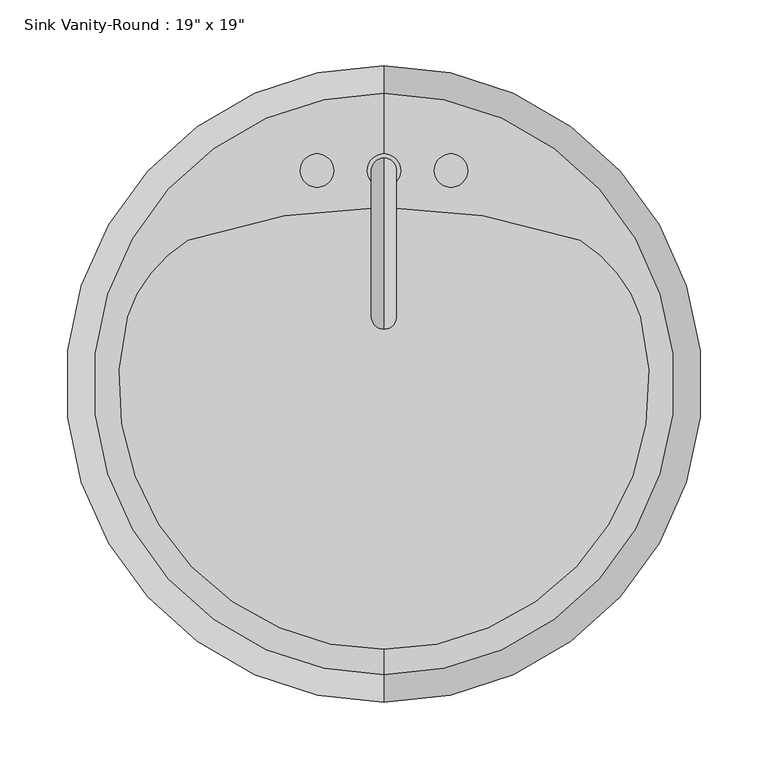
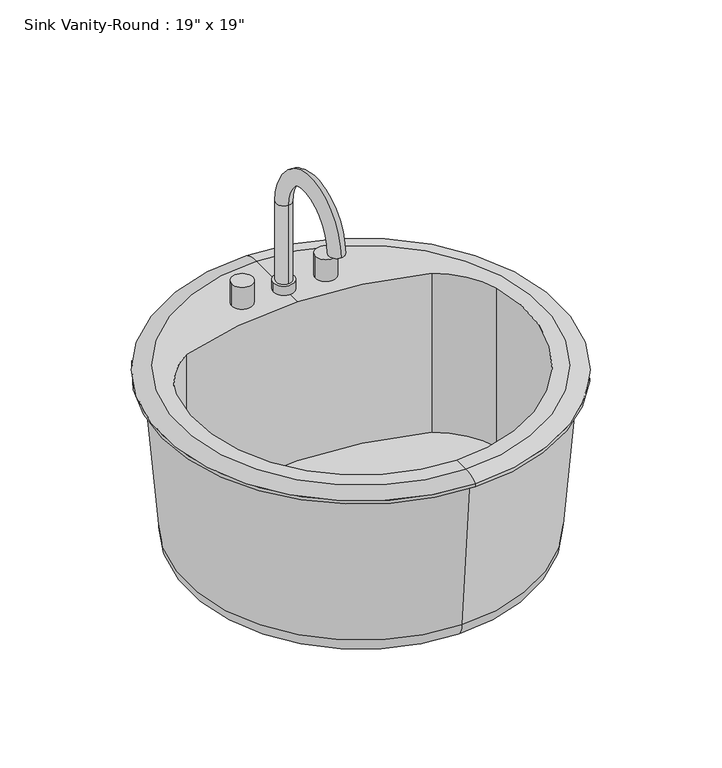
"""IFC4 building model written with IfcOpenShell, lengths in millimetres: flow terminal geometry."""

from ifc_helpers import new_model, si_unit, point, frame, frame_2d, origin, place, context, project, spatial, polyline, circle_curve, ellipse_curve, trimmed, segment, composite_curve, outline, extrude, source, transform, mapped, element, save
from ifc_brep_helpers import plane_surface, cylinder_surface, revolved_surface, advanced_brep


def flow_terminal_a43f4bde(model_context):
    return source(origin(), model_context, "Body", "SolidModel", [
        advanced_brep(
        [(96.6517406, -135.3870093, 796.925), (96.6517406, 305.7224463, 796.925), (96.6517406, 326.4677185, 791.36875), (96.6517406, -156.1322815, 791.36875), (96.6517406, -116.2405705, 796.925), (-98.1703414, 136.2525038, 796.925), (-52.1534933, 194.0861398, 796.925), (96.6517406, 219.2662048, 796.925), (245.4569744, 194.0861398, 796.925), (291.4738225, 136.2525038, 796.925), (96.6517406, -107.1264028, 571.5), (96.6517406, 277.4618398, 571.5), (96.6517406, 85.1677185, 571.5), (96.6517406, -127.6827361, 592.6842611), (96.6517406, 298.0181731, 592.6842611), (96.6517406, -144.2260315, 787.4), (96.6517406, 314.5614685, 787.4), (96.6517406, -156.1322815, 787.4), (96.6517406, 326.4677185, 787.4), (245.4569744, 194.0861398, 592.6842611), (-52.1534933, 194.0861398, 592.6842611), (-98.1703414, 136.2525038, 592.6842611), (291.4738225, 136.2525038, 592.6842611)],
        [
            (0, 1, circle_curve(frame((96.6517406, 85.1677185, 796.925), z_axis=(0.0, 0.0, -1.0), x_axis=(0.0, 1.0, 0.0)), 220.5547278)),
            (1, 2, circle_curve(frame((96.6517406, 309.4374616, 769.289434), z_axis=(-1.0, 0.0, 0.0), x_axis=(0.0, 1.0, 0.0)), 27.8841505)),
            (2, 3, circle_curve(frame((96.6517406, 85.1677185, 791.36875), z_axis=(0.0, 0.0, 1.0), x_axis=(0.0, 1.0, 0.0)), 241.3)),
            (3, 0, circle_curve(frame((96.6517406, -139.1020246, 769.289434), z_axis=(-1.0, 0.0, 0.0), x_axis=(0.0, -1.0, 0.0)), 27.8841505)),
            (1, 0, circle_curve(frame((96.6517406, 85.1677185, 796.925), z_axis=(0.0, 0.0, -1.0), x_axis=(0.0, 1.0, 0.0)), 220.5547278)),
            (3, 2, circle_curve(frame((96.6517406, 85.1677185, 791.36875), z_axis=(0.0, 0.0, 1.0), x_axis=(0.0, 1.0, 0.0)), 241.3)),
            (0, 4),
            (4, 5, circle_curve(frame((96.6517406, 85.1677185, 796.925), z_axis=(0.0, 0.0, -1.0), x_axis=(1.0, 0.0, 0.0)), 201.408289)),
            (5, 6, circle_curve(frame((1.3689689, 104.2755165, 796.925), z_axis=(0.0, 0.0, -1.0), x_axis=(1.0, 0.0, 0.0)), 104.5495194)),
            (6, 7, circle_curve(frame((96.6517406, -233.0168462, 796.925), z_axis=(0.0, 0.0, -1.0), x_axis=(1.0, 0.0, 0.0)), 452.283051)),
            (7, 1),
            (7, 8, circle_curve(frame((96.6517406, -233.0168462, 796.925), z_axis=(0.0, 0.0, -1.0), x_axis=(1.0, 0.0, 0.0)), 452.283051)),
            (8, 9, circle_curve(frame((191.9345122, 104.2755165, 796.925), z_axis=(0.0, 0.0, -1.0), x_axis=(1.0, 0.0, 0.0)), 104.5495194)),
            (9, 4, circle_curve(frame((96.6517406, 85.1677185, 796.925), z_axis=(0.0, 0.0, -1.0), x_axis=(1.0, 0.0, 0.0)), 201.408289)),
            (10, 11, circle_curve(frame((96.6517406, 85.1677185, 571.5), z_axis=(0.0, 0.0, -1.0), x_axis=(0.0, 1.0, 0.0)), 192.2941213)),
            (11, 12),
            (12, 10),
            (11, 10, circle_curve(frame((96.6517406, 85.1677185, 571.5), z_axis=(0.0, 0.0, -1.0), x_axis=(0.0, 1.0, 0.0)), 192.2941213)),
            (10, 13, circle_curve(frame((96.6517406, -107.1264028, 592.0656396), z_axis=(-1.0, 0.0, 0.0), x_axis=(0.0, -1.0, 0.0)), 20.5656396)),
            (13, 14, circle_curve(frame((96.6517406, 85.1677185, 592.6842611), z_axis=(0.0, 0.0, -1.0), x_axis=(0.0, 1.0, 0.0)), 212.8504546)),
            (14, 11, circle_curve(frame((96.6517406, 277.4618398, 592.0656396), z_axis=(-1.0, 0.0, 0.0), x_axis=(0.0, 1.0, 0.0)), 20.5656396)),
            (14, 13, circle_curve(frame((96.6517406, 85.1677185, 592.6842611), z_axis=(0.0, 0.0, -1.0), x_axis=(0.0, 1.0, 0.0)), 212.8504546)),
            (13, 15),
            (15, 16, circle_curve(frame((96.6517406, 85.1677185, 787.4), z_axis=(0.0, 0.0, -1.0), x_axis=(0.0, 1.0, 0.0)), 229.39375)),
            (16, 14),
            (16, 15, circle_curve(frame((96.6517406, 85.1677185, 787.4), z_axis=(0.0, 0.0, -1.0), x_axis=(0.0, 1.0, 0.0)), 229.39375)),
            (15, 17),
            (17, 18, circle_curve(frame((96.6517406, 85.1677185, 787.4), z_axis=(0.0, 0.0, -1.0), x_axis=(0.0, 1.0, 0.0)), 241.3)),
            (18, 16),
            (18, 17, circle_curve(frame((96.6517406, 85.1677185, 787.4), z_axis=(0.0, 0.0, -1.0), x_axis=(0.0, 1.0, 0.0)), 241.3)),
            (2, 18),
            (17, 3),
            (19, 20, circle_curve(frame((96.6517406, -233.0168462, 592.6842611), z_axis=(0.0, 0.0, 1.0), x_axis=(1.0, 0.0, 0.0)), 452.283051)),
            (20, 21, circle_curve(frame((1.3689689, 104.2755165, 592.6842611), z_axis=(0.0, 0.0, 1.0), x_axis=(1.0, 0.0, 0.0)), 104.5495194)),
            (21, 22, circle_curve(frame((96.6517406, 85.1677185, 592.6842611), z_axis=(0.0, 0.0, 1.0), x_axis=(1.0, 0.0, 0.0)), 201.408289)),
            (22, 19, circle_curve(frame((191.9345122, 104.2755165, 592.6842611), z_axis=(0.0, 0.0, 1.0), x_axis=(1.0, 0.0, 0.0)), 104.5495194)),
            (19, 8),
            (6, 20),
            (5, 21),
            (9, 22),
        ],
        [
            revolved_surface(trimmed(ellipse_curve(frame((96.6517406, 309.4374616, 769.289434), z_axis=(1.0, 0.0, 0.0), x_axis=(0.0, 1.0, 0.0)), 27.8841505, 27.8841505), [point((96.6517406, 326.4677185, 791.36875))], [point((96.6517406, 305.7224463, 796.925))], True, "CARTESIAN"), (96.6517406, 85.1677185, 796.925), (0.0, 0.0, 1.0)),
            plane_surface(frame((96.6517406, 85.1677185, 796.925), z_axis=(0.0, 0.0, 1.0), x_axis=(0.0, 1.0, 0.0))),
            plane_surface(frame((96.6517406, 85.1677185, 571.5), z_axis=(0.0, 0.0, -1.0), x_axis=(0.0, 1.0, 0.0))),
            revolved_surface(trimmed(ellipse_curve(frame((96.6517406, 277.4618398, 592.0656396), z_axis=(1.0, 0.0, 0.0), x_axis=(0.0, 1.0, 0.0)), 20.5656396, 20.5656396), [point((96.6517406, 277.4618398, 571.5))], [point((96.6517406, 298.0181731, 592.6842611))], True, "CARTESIAN"), (96.6517406, 85.1677185, 796.925), (0.0, 0.0, 1.0)),
            revolved_surface(polyline([(96.6517406, 298.0181731, 592.6842611), (96.6517406, 314.5614685, 787.4)]), (96.6517406, 85.1677185, 796.925), (0.0, 0.0, 1.0)),
            plane_surface(frame((96.6517406, 85.1677185, 787.4), z_axis=(0.0, 0.0, -1.0), x_axis=(0.0, 1.0, 0.0))),
            cylinder_surface(frame((96.6517406, 85.1677185, 796.925), z_axis=(0.0, 0.0, 1.0), x_axis=(0.0, 1.0, 0.0)), 241.3),
            plane_surface(frame((548.9347916, -233.0168462, 592.6842611), z_axis=(0.0, 0.0, 1.0), x_axis=(0.0, -1.0, 0.0))),
            revolved_surface(polyline([(548.9347916, -233.0168462, 796.925), (548.9347916, -233.0168462, 592.6842611)]), (96.6517406, -233.0168462, 592.6842611), (0.0, 0.0, 1.0)),
            revolved_surface(polyline([(105.91848829999999, 104.2755165, 796.925), (105.91848829999999, 104.2755165, 592.6842611)]), (1.3689689, 104.2755165, 592.6842611), (0.0, 0.0, 1.0)),
            revolved_surface(polyline([(298.0600296, 85.1677185, 796.925), (298.0600296, 85.1677185, 592.6842611)]), (96.6517406, 85.1677185, 592.6842611), (0.0, 0.0, 1.0)),
            revolved_surface(polyline([(296.4840316, 104.2755165, 796.925), (296.4840316, 104.2755165, 592.6842611)]), (191.9345122, 104.2755165, 592.6842611), (0.0, 0.0, 1.0)),
        ],
        [
            (0, [[1, 2, 3, 4]]),
            (0, [[-2, 5, -4, 6]]),
            (1, [[-1, 7, 8, 9, 10, 11]]),
            (1, [[-5, -11, 12, 13, 14, -7]]),
            (2, [[15, 16, 17]]),
            (2, [[-16, 18, -17]]),
            (3, [[-15, 19, 20, 21]]),
            (3, [[-18, -21, 22, -19]]),
            (4, [[-20, 23, 24, 25]]),
            (4, [[-22, -25, 26, -23]]),
            (5, [[-24, 27, 28, 29]]),
            (5, [[-26, -29, 30, -27]]),
            (6, [[-3, 31, -28, 32]]),
            (6, [[-6, -32, -30, -31]]),
            (7, [[33, 34, 35, 36]]),
            (8, [[-33, 37, -12, -10, 38]]),
            (9, [[-34, -38, -9, 39]]),
            (10, [[-35, -39, -8, -14, 40]]),
            (11, [[-36, -40, -13, -37]]),
        ],
    ),
        extrude(outline(composite_curve([segment(trimmed(circle_curve(frame_2d((96.6517406, 85.1677185)), 20.6375), [point((76.0142406, 85.1677185))], [point((117.2892406, 85.1677185))], False, "CARTESIAN"), True, "CONTINUOUS"), segment(trimmed(circle_curve(frame_2d((96.6517406, 85.1677185)), 20.6375), [point((117.2892406, 85.1677185))], [point((76.0142406, 85.1677185))], False, "CARTESIAN"), True, "CONTINUOUS")], self_intersect=False)), frame((0.0, 0.0, 571.5), z_axis=(0.0, 0.0, 1.0), x_axis=(1.0, 0.0, 0.0)), (0.0, 0.0, 1.0), 21.1842611),
        extrude(outline(composite_curve([segment(trimmed(circle_curve(frame_2d((147.4517406, 247.0927185)), 12.7), [point((134.7517406, 247.0927185))], [point((160.1517406, 247.0927185))], False, "CARTESIAN"), True, "CONTINUOUS"), segment(trimmed(circle_curve(frame_2d((147.4517406, 247.0927185)), 12.7), [point((160.1517406, 247.0927185))], [point((134.7517406, 247.0927185))], False, "CARTESIAN"), True, "CONTINUOUS")], self_intersect=False)), frame((0.0, 0.0, 796.925), z_axis=(0.0, 0.0, 1.0), x_axis=(1.0, 0.0, 0.0)), (0.0, 0.0, 1.0), 28.575),
        extrude(outline(composite_curve([segment(trimmed(circle_curve(frame_2d((45.8517406, 247.0927185)), 12.7), [point((33.1517406, 247.0927185))], [point((58.5517406, 247.0927185))], False, "CARTESIAN"), True, "CONTINUOUS"), segment(trimmed(circle_curve(frame_2d((45.8517406, 247.0927185)), 12.7), [point((58.5517406, 247.0927185))], [point((33.1517406, 247.0927185))], False, "CARTESIAN"), True, "CONTINUOUS")], self_intersect=False)), frame((0.0, 0.0, 796.925), z_axis=(0.0, 0.0, 1.0), x_axis=(1.0, 0.0, 0.0)), (0.0, 0.0, 1.0), 28.575),
        advanced_brep(
        [(83.9517406, 247.0927185, 796.925), (109.3517406, 247.0927185, 796.925), (96.6517406, 237.5677185, 909.6375), (96.6517406, 256.6177185, 909.6375), (96.6517406, 256.6177185, 809.1602909), (96.6517406, 237.5677185, 809.1602909), (96.6517406, 145.7775038, 909.6375), (96.6517406, 126.7275038, 909.6375), (83.9517406, 247.0927185, 809.1602909), (109.3517406, 247.0927185, 809.1602909)],
        [
            (0, 1, circle_curve(frame((96.6517406, 247.0927185, 796.925), z_axis=(0.0, 0.0, -1.0), x_axis=(1.0, 0.0, 0.0)), 12.7)),
            (1, 0, circle_curve(frame((96.6517406, 247.0927185, 796.925), z_axis=(0.0, 0.0, -1.0), x_axis=(1.0, 0.0, 0.0)), 12.7)),
            (2, 3, circle_curve(frame((96.6517406, 247.0927185, 909.6375), z_axis=(0.0, 0.0, -1.0), x_axis=(0.0, 1.0, 0.0)), 9.525)),
            (3, 4),
            (4, 5, circle_curve(frame((96.6517406, 247.0927185, 809.1602909), z_axis=(0.0, 0.0, 1.0), x_axis=(0.0, 1.0, 0.0)), 9.525)),
            (5, 2),
            (3, 2, circle_curve(frame((96.6517406, 247.0927185, 909.6375), z_axis=(0.0, 0.0, -1.0), x_axis=(0.0, 1.0, 0.0)), 9.525)),
            (5, 4, circle_curve(frame((96.6517406, 247.0927185, 809.1602909), z_axis=(0.0, 0.0, 1.0), x_axis=(0.0, 1.0, 0.0)), 9.525)),
            (6, 7, circle_curve(frame((96.6517406, 136.2525038, 909.6375), z_axis=(0.0, 0.0, -1.0), x_axis=(0.0, -1.0, 0.0)), 9.525)),
            (7, 6, circle_curve(frame((96.6517406, 136.2525038, 909.6375), z_axis=(0.0, 0.0, -1.0), x_axis=(0.0, -1.0, 0.0)), 9.525)),
            (2, 6, circle_curve(frame((96.6517406, 191.6726112, 909.6375), z_axis=(1.0, 0.0, 0.0), x_axis=(0.0, 1.0, 0.0)), 45.8951073)),
            (7, 3, circle_curve(frame((96.6517406, 191.6726112, 909.6375), z_axis=(-1.0, 0.0, 0.0), x_axis=(0.0, 1.0, 0.0)), 64.9451073)),
            (8, 9, circle_curve(frame((96.6517406, 247.0927185, 809.1602909), z_axis=(0.0, 0.0, 1.0), x_axis=(1.0, 0.0, 0.0)), 12.7)),
            (9, 8, circle_curve(frame((96.6517406, 247.0927185, 809.1602909), z_axis=(0.0, 0.0, 1.0), x_axis=(1.0, 0.0, 0.0)), 12.7)),
            (8, 0),
            (1, 9),
        ],
        [
            plane_surface(frame((96.6517406, 237.5677185, 796.925), z_axis=(0.0, 0.0, -1.0), x_axis=(1.0, 0.0, 0.0))),
            cylinder_surface(frame((96.6517406, 247.0927185, 796.925), z_axis=(0.0, 0.0, -1.0), x_axis=(0.0, 1.0, 0.0)), 9.525),
            plane_surface(frame((96.6517406, 191.6726112, 909.6375), z_axis=(0.0, 0.0, -1.0), x_axis=(0.0, -1.0, 0.0))),
            revolved_surface(trimmed(ellipse_curve(frame((96.6517406, 247.0927185, 909.6375), z_axis=(0.0, 0.0, -1.0), x_axis=(0.0, 1.0, 0.0)), 9.525, 9.525), [point((96.6517406, 237.5677185, 909.6375))], [point((96.6517406, 256.6177185, 909.6375))], True, "CARTESIAN"), (96.6517406, 191.6726112, 909.6375), (1.0, 0.0, 0.0)),
            revolved_surface(trimmed(ellipse_curve(frame((96.6517406, 247.0927185, 909.6375), z_axis=(0.0, 0.0, -1.0), x_axis=(0.0, 1.0, 0.0)), 9.525, 9.525), [point((96.6517406, 256.6177185, 909.6375))], [point((96.6517406, 237.5677185, 909.6375))], True, "CARTESIAN"), (96.6517406, 191.6726112, 909.6375), (1.0, 0.0, 0.0)),
            plane_surface(frame((109.3517406, 247.0927185, 809.1602909), z_axis=(0.0, 0.0, 1.0), x_axis=(0.0, 1.0, 0.0))),
            cylinder_surface(frame((96.6517406, 247.0927185, 796.925), z_axis=(0.0, 0.0, 1.0), x_axis=(1.0, 0.0, 0.0)), 12.7),
        ],
        [
            (0, [[1, 2]]),
            (1, [[3, 4, 5, 6]]),
            (1, [[7, -6, 8, -4]]),
            (2, [[9, 10]]),
            (3, [[-3, 11, -10, 12]]),
            (4, [[-7, -12, -9, -11]]),
            (5, [[13, 14], [-5, -8]]),
            (6, [[-13, 15, -2, 16]]),
            (6, [[-14, -16, -1, -15]]),
        ],
    ),
    ])


if __name__ == "__main__":
    model = new_model("IFC4")
    model_context = context("Model", 3, world=origin())
    ifc_project = project(units=[si_unit("LENGTHUNIT", "METRE", prefix="MILLI")], contexts=[model_context])
    site = spatial("IfcSite", under=ifc_project)
    building = spatial("IfcBuilding", under=site)
    placement = place(None, origin())
    flow_terminal_shape = flow_terminal_a43f4bde(model_context)
    element("IfcFlowTerminal", 1, ObjectType="Sink Vanity-Round : 19\" x 19\"", at=placement, inside=building, context=model_context, shape_type="MappedRepresentation", body=[
        mapped(flow_terminal_shape, transform((0.0, 0.0, 0.0), x_axis=(1.0, 0.0, 0.0), y_axis=(0.0, 1.0, 0.0), z_axis=(0.0, 0.0, 1.0))),
    ])
    save(model, "model.ifc")

# Revit data of these elements
# Type "Sink Vanity-Round : 19\" x 19\""
#   Assembly Code = "D2010400"
#   Top Of Counter = 787.4 mm
#   Basin Material = Porcelain, Linen
#   Faucet Material = Steel, Polished
#   Default Elevation = 0
# Element 1 (IfcFlowTerminal, "Sink Vanity-Round : 19\" x 19\"")
#   Materials on its faces: "Porcelain, Linen", "Steel, Polished"
# Materials
#   "Porcelain, Linen": class "Ceramic", colour RGB 249 239 230, transparency 0, Description = "Porcelain, linen", Cost = 0
#   "Steel, Polished": class "Metal", colour RGB 57 57 57, transparency 0, Description = "Polished steel", Cost = 0
